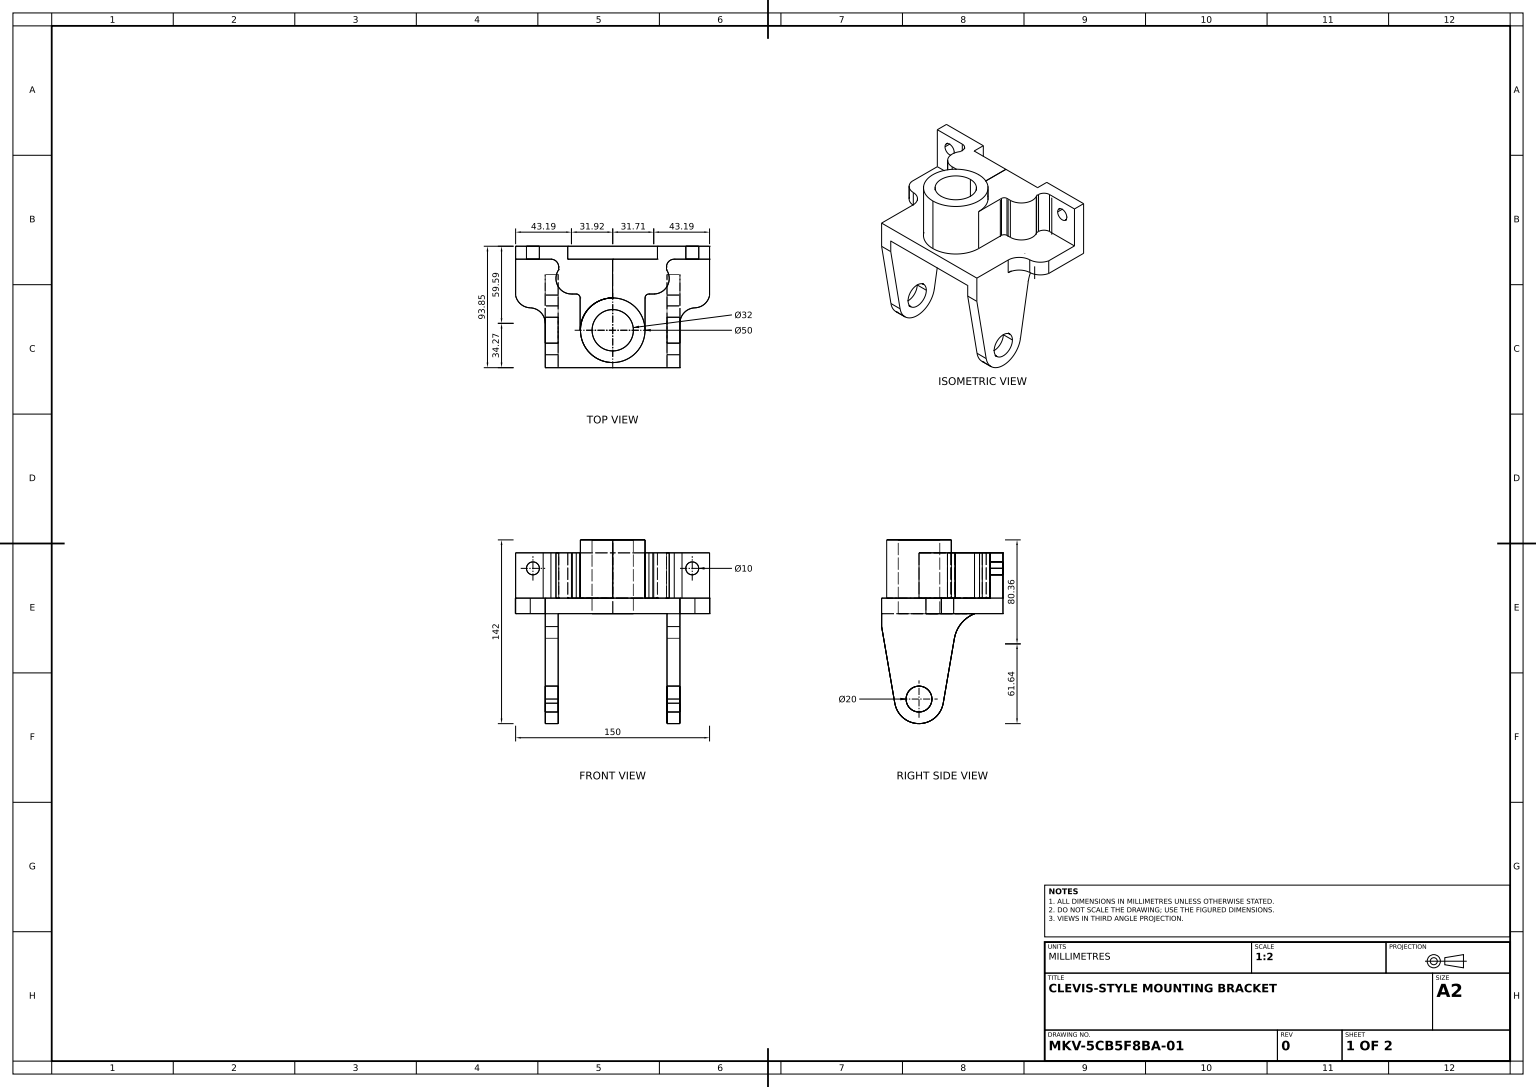
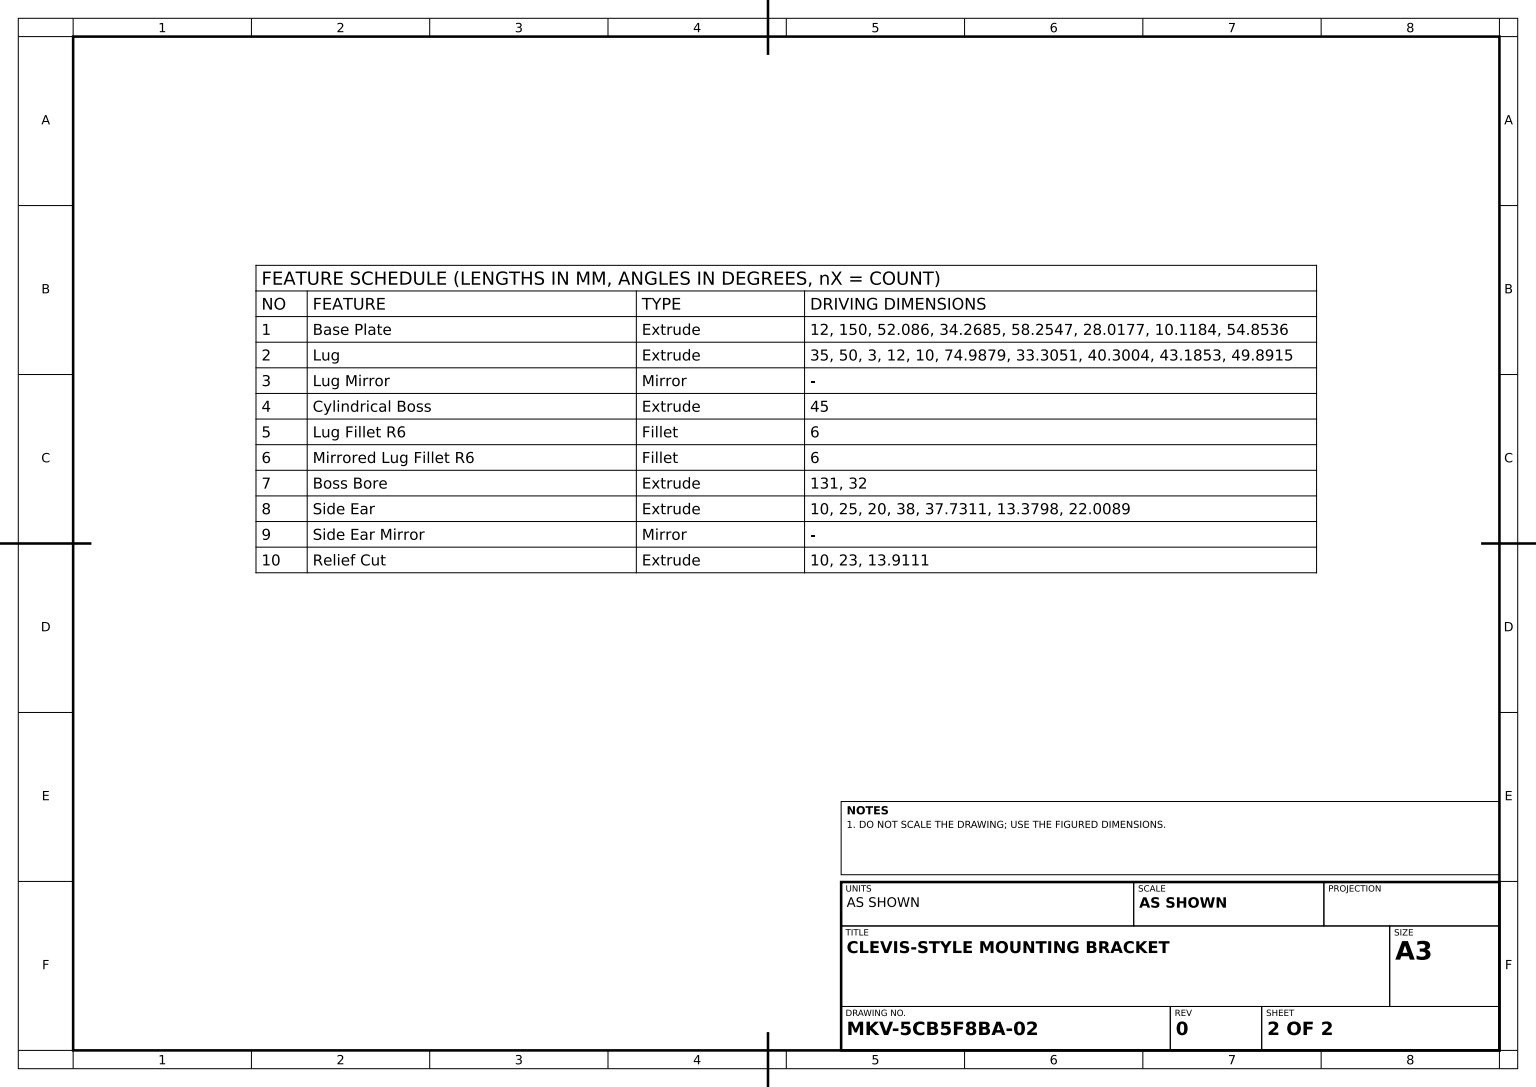
SolidWorks part; units mm, degrees
material "Plain Carbon Steel"
ref_plane "Front Plane" through (0, 0, 0) normal (0, 0, 1) x (1, 0, 0)
ref_plane "Top Plane" through (0, 0, 0) normal (0, 1, 0) x (1, 0, 0)
ref_plane "Right Plane" through (0, 0, 0) normal (1, 0, 0) x (0, 0, -1)
sketch "Base Plate Sketch" plane through (0, 0, 0) normal (0, 1, 0) x (1, 0, 0)
  line L1 (0, 0) -> (52.086, 0)
  line L2 (52.086, 0) -> (52.086, 34.2685)
  line L3 (75, 55.7177) -> (75, 83.7354)
  line L4 (75, 83.7354) -> (75, 93.8538)
  line L5 (75, 93.8538) -> (20.1464, 93.8538)
  line L6 (-52.086, 0) -> (-52.086, 34.2685)
  line L7 (-75, 83.7354) -> (-75, 93.8538)
  line L8 (-75, 55.7177) -> (-75, 83.7354)
  line L9 (-75, 93.8538) -> (20.1464, 93.8538)
  line L10 (-52.086, 0) -> (0, 0)
  arc A0 (52.086, 34.2685) -> (63.6786, 46.2616) centre (64.086, 34.2685) cw
  arc A1 (63.6786, 46.2616) -> (75, 55.7177) centre (63.2712, 58.2547) ccw
  arc A2 (-52.086, 34.2685) -> (-63.6786, 46.2616) centre (-64.086, 34.2685) ccw
  arc A3 (-63.6786, 46.2616) -> (-75, 55.7177) centre (-63.2712, 58.2547) cw
  point P4 (0, 0)
  dimension "D1" = 150
  dimension "D2" = 12
  dimension "D3" = 12
  dimension "D7" = 28.0177
  dimension "D4" = 52.086
  dimension "D5" = 34.2685
  dimension "D6" = 58.2547
  dimension "D8" = 10.1184
  dimension "D9" = 54.8536
extrude "Base Plate" add sketch "Base Plate Sketch" along normal blind 12
sketch "Lug Sketch" plane through (0, 12, 0) normal (0, 1, 0) x (1, 0, 0)
  line L0 (25.1085, 28.9239) -> (25.1085, 53.9239)
  line L1 (28.1085, 56.9239) -> (31.8147, 56.9239)
  line L2 (41.6949, 75.7343) -> (41.6949, 83.8538)
  line L3 (41.6949, 83.8538) -> (75, 83.8538)
  line L4 (75, 55.7177) -> (75, 93.8538) construction
  line L5 (75, 83.8538) -> (75, 93.8538)
  line L6 (75, 93.8538) -> (-75, 93.8538) construction
  line L7 (75, 93.8538) -> (41.6949, 93.8538)
  line L8 (0, 93.8538) -> (0.1085, 3.9239)
  line L9 (41.6949, 93.8538) -> (34.6996, 93.8538)
  line L10 (34.6996, 93.8538) -> (34.6996, 83.8538)
  line L11 (34.6996, 83.8538) -> (0.0121, 83.8538)
  circle A0 centre (0.1085, 28.9239) radius 25
  arc A1 (25.1085, 53.9239) -> (28.1085, 56.9239) centre (28.1085, 53.9239) cw
  arc A2 (31.8147, 56.9239) -> (41.6949, 75.7343) centre (31.8147, 68.9239) ccw
  dimension "D1" = 50
  dimension "D2" = 3
  dimension "D3" = 12
  dimension "D4" = 10
  dimension "D5" = 33.3051
  dimension "D6" = 40.3004
  dimension "D7" = 43.1853
  dimension "D8" = 49.8915
  dimension "D10" = 74.9879
extrude "Lug" add sketch "Lug Sketch" along normal blind 35
mirror "Lug Mirror" about plane through (0, 0, 0) normal (1, 0, 0) of "Lug"
sketch "Boss Sketch" plane through (0, 12, 0) normal (0, 1, 0) x (1, 0, 0)
  circle A0 centre (0.1085, 28.9239) radius 25
extrude "Cylindrical Boss" add sketch "Boss Sketch" along normal blind 45
fillet "Lug Fillet R6" radius 6 1 edges at (41.6949, 29.5, -83.8538)
fillet "Mirrored Lug Fillet R6" radius 6 1 edges at (-41.6949, 29.5, -83.8538)
sketch "Boss Bore Sketch" plane through (0, 57, 0) normal (0, 1, 0) x (1, 0, 0)
  circle A0 centre (0.1085, 28.9239) radius 16
  dimension "D1" = 32
extrude "Boss Bore" cut sketch "Boss Bore Sketch" against normal blind 131
sketch "Side Ear Sketch" plane through (52.086, 0, 0) normal (1, 0, 0) x (0, 0, -1)
  line L0 (0, 0) -> (0, -9.9939)
  line L1 (28.9239, 57) -> (28.9239, 0)
  line L2 (34.2685, 12) -> (34.2685, 0) construction
  line L3 (44.9239, 57) -> (12.9239, 57) construction
  line L4 (0, 0) -> (34.2685, 0) construction
  line L5 (28.9239, 0) -> (28.9239, -66) construction
  line L6 (10.1995, -69.2243) -> (0, -9.9939)
  line L7 (47.6483, -69.2243) -> (56.2773, -19.1138)
  line L8 (55.7177, 0) -> (93.8538, 0) construction
  line L9 (46.2616, 0) -> (55.7177, 0) construction
  line L10 (34.2685, 0) -> (46.2616, 0) construction
  line L11 (55.7177, 0) -> (71.9996, 0)
  line L12 (46.2616, 0) -> (55.7177, 0)
  line L13 (0, 0) -> (34.2685, 0)
  line L14 (34.2685, 0) -> (46.2616, 0)
  circle A0 centre (28.9239, -66) radius 19
  arc A1 (56.2773, -19.1138) -> (71.9996, 0) centre (80.9147, -23.3564) cw
  circle A2 centre (28.9239, -66) radius 10
  dimension "D1" = 25
  dimension "D2" = 20
  dimension "D3" = 38
  dimension "D4" = 13.3798
  dimension "D5" = 22.0089
  dimension "D6" = 37.7311
extrude "Side Ear" add sketch "Side Ear Sketch" against normal blind 10
mirror "Side Ear Mirror" about plane through (0, 0, 0) normal (1, 0, 0) of "Side Ear"
sketch "Relief Cut Sketch" plane through (0, 0, -83.8538) normal (0, 0, 1) x (1, 0, 0)
  line L0 (0, -51.6196) -> (0, 51.6196) construction
  line L1 (47.6949, 47) -> (47.6949, 12) construction
  circle A0 centre (61.606, 35) radius 5
  circle A1 centre (-61.606, 35) radius 5
  dimension "D1" = 23
  dimension "D2" = 10
  dimension "D3" = 13.9111
extrude "Relief Cut" cut sketch "Relief Cut Sketch" against normal blind 10
